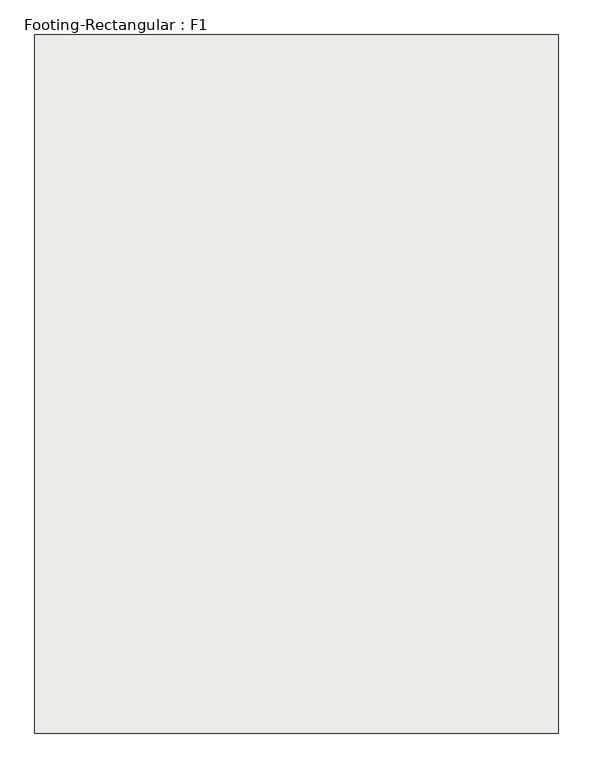
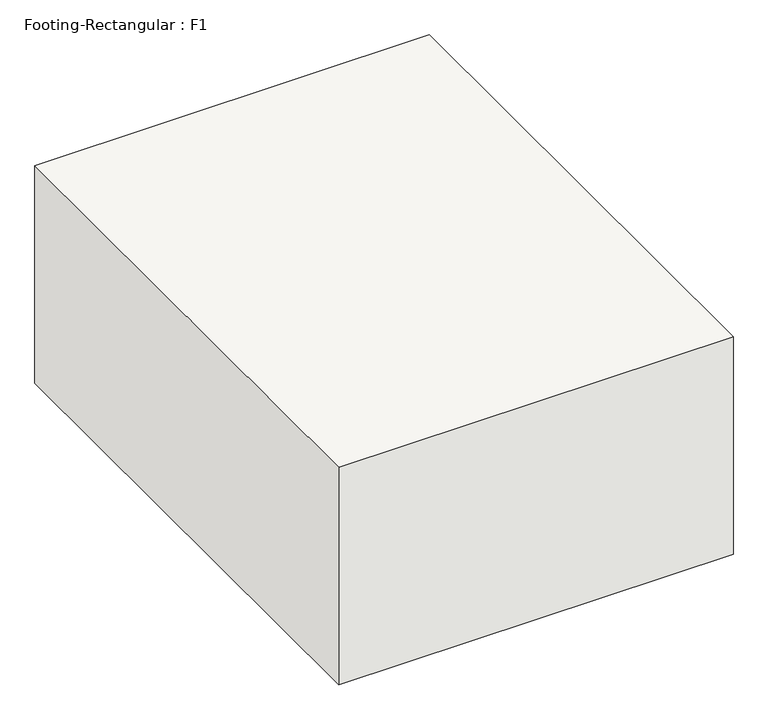
"""IFC4 building model written with IfcOpenShell, lengths in millimetres: slab geometry, Footing-Rectangular : F1."""

from ifc_helpers import new_model, si_unit, frame, origin, place, context, project, spatial, polyline, outline, extrude, source, transform, mapped, element, save


def footing_rectangular_f1_21e6a39c(model_context):
    return source(origin(), model_context, "Body", "SweptSolid", [
        extrude(outline(polyline([(457.2, 609.6), (457.2, -609.6), (-457.2, -609.6), (-457.2, 609.6), (457.2, 609.6)])), frame((0.0, 0.0, -533.4), z_axis=(0.0, 0.0, 1.0), x_axis=(1.0, 0.0, 0.0)), (0.0, 0.0, 1.0), 533.4),
    ])


if __name__ == "__main__":
    model = new_model("IFC4")
    model_context = context("Model", 3, world=origin())
    ifc_project = project(units=[si_unit("LENGTHUNIT", "METRE", prefix="MILLI")], contexts=[model_context])
    site = spatial("IfcSite", under=ifc_project)
    building = spatial("IfcBuilding", under=site)
    placement = place(None, origin())
    footing_rectangular_f1_shape = footing_rectangular_f1_21e6a39c(model_context)
    element("IfcSlab", 1, ObjectType="Footing-Rectangular : F1", at=placement, inside=building, context=model_context, shape_type="MappedRepresentation", body=[
        mapped(footing_rectangular_f1_shape, transform((0.0, 0.0, 0.0), x_axis=(1.0, 0.0, 0.0), y_axis=(0.0, 1.0, 0.0), z_axis=(0.0, 0.0, 1.0))),
    ])
    save(model, "model.ifc")

# Revit data of these elements
# Type "Footing-Rectangular : F1"
#   Width = 914.4 mm
#   Length = 1219.2 mm
#   Foundation Thickness = 533.4 mm
#   Structural Material [instance default] = Concrete - Cast-in-Place Concrete
#   Assembly Code = ""
# Element 1 (IfcSlab, "Footing-Rectangular : F1")
#   Materials on its faces: "Concrete - Cast-in-Place Concrete"
# Materials
#   "Concrete - Cast-in-Place Concrete": class "Concrete", colour RGB 192 192 192, transparency 0, Cost = 0
